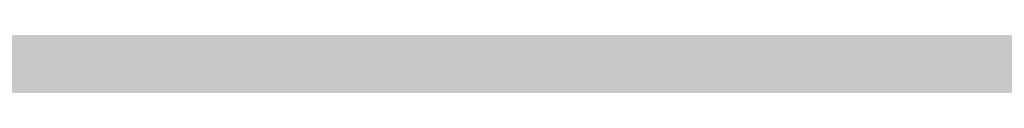
# Model space of a CAD drawing. Units: inches. Extents: x 2091 to 2899, y 967 to 2217.
# Tile 185 of 256: x 2203.16122 to 2203.18039, y 1152.2479 to 1152.24874. Entities that reach past the tile are written whole.
import ezdxf

# ---------------------------------------------------------------- set-up
doc = ezdxf.new("R2010")
doc.units = ezdxf.units.IN
doc.layers.add('A-WALL-PATT', color=141, linetype='Continuous', lineweight=13, true_color=0xadddf7)

msp = doc.modelspace()

# ---------------------------------------------------------------- hatches: boundary and pattern name
at = {"layer": 'A-WALL-PATT'}
h = msp.add_hatch(color=256, dxfattribs=at)
h.dxf.hatch_style = 1
h.paths.add_polyline_path([(2803.143603, 2050.919059), (2203.143603, 2050.919059), (2203.143603, 1090.919059), (2803.143603, 1090.919059)])
h.paths.add_polyline_path([(2635.79885, 1147.540465), (2674.524052, 1147.540465, 0.376086), (2678.529665, 1152.880202), (2678.529665, 1159.556473, 0.333335), (2674.524319, 1163.561846), (2674.524319, 1163.56185), (2674.524319, 1192.93439), (2635.805971, 1192.93439), (2597.087622, 1192.93439), (2597.087622, 1163.561846, 0.333335), (2593.082276, 1159.556473), (2593.082276, 1152.880202, 0.376086), (2597.087889, 1147.540465)], flags=0)
h.paths.add_polyline_path([(2436.010433, 1278.240778, 0.000483), (2435.952643, 1278.215027, -0.001328), (2435.935625, 1278.111693, -0.001711), (2436.11644, 1278.040758, 0.002185)], flags=0)
h.paths.add_polyline_path([(2794.143603, 1143.419059), (2794.143603, 1347.419059), (2543.370171, 1347.419059), (2543.370171, 1351.919059), (2794.143603, 1351.919059), (2794.143603, 1392.713555), (2793.947398, 1392.713555), (2793.947398, 1473.5369), (2794.143603, 1473.5369), (2794.143603, 1531.919059), (2650.143603, 1531.919059), (2650.143603, 1536.419059), (2794.143603, 1536.419059), (2794.143603, 1692.419059), (2609.375609, 1692.419059), (2609.375609, 1644.419059), (2604.875609, 1644.419059), (2604.875609, 1744.919059), (2609.375609, 1744.919059), (2609.375609, 1696.919059), (2794.143603, 1696.919059), (2794.143603, 1780.919059), (2609.643603, 1780.919059), (2493.875609, 1780.919059), (2493.875609, 1785.419059), (2609.643603, 1785.419059), (2794.143603, 1785.419059), (2794.143603, 1847.938821), (2793.951222, 1847.938821), (2793.951222, 1928.762166), (2794.143603, 1928.762166), (2794.143603, 1941.419059), (2614.143603, 1941.419059), (2614.143603, 1821.419059), (2609.643603, 1821.419059), (2609.643603, 1941.419059), (2392.143603, 1941.419059), (2392.143603, 1819.919059), (2387.643603, 1819.919059), (2387.643603, 1941.419059), (2212.143603, 1941.419059), (2212.143603, 1783.919059), (2392.143603, 1783.919059), (2392.143603, 1780.919059), (2212.143603, 1780.919059), (2212.143603, 1629.419059), (2387.643603, 1629.419059), (2387.643603, 1744.919059), (2392.143603, 1744.919059), (2392.143603, 1627.919059), (2317.143603, 1627.919059), (2317.143603, 1551.419059), (2317.143603, 1536.419059), (2459.383591, 1536.419059), (2459.383591, 1602.39648), (2463.883591, 1602.39648), (2463.883591, 1531.919059), (2456.643603, 1531.919059), (2456.643603, 1529.919059), (2452.143603, 1529.919059), (2452.143603, 1531.919059), (2312.643603, 1531.919059), (2312.643603, 1551.419059), (2306.143603, 1551.419059), (2306.143603, 1555.919059), (2308.143603, 1555.919059), (2308.143603, 1551.419059), (2312.643603, 1551.419059), (2312.643603, 1627.919059), (2212.143603, 1627.919059), (2212.143603, 1555.919059), (2270.143603, 1555.919059), (2270.143603, 1551.419059), (2212.143603, 1551.419059), (2212.143603, 1351.919059), (2272.143603, 1351.919059), (2272.143603, 1347.419059), (2212.143603, 1347.419059), (2212.143603, 1275.419059), (2308.143603, 1275.419059), (2308.143603, 1351.919059), (2452.143603, 1351.919059), (2452.143603, 1493.919059), (2456.643603, 1493.919059), (2456.643603, 1347.419059), (2312.643603, 1347.419059), (2312.643603, 1270.919059), (2212.143603, 1270.919059), (2212.143603, 1099.919059), (2281.237523, 1099.919059), (2282.871041, 1110.913803), (2282.008341, 1116.996603), (2278.557741, 1121.420403), (2268.205641, 1128.056203), (2272.087641, 1128.056203), (2273.812941, 1131.927003), (2279.420341, 1134.691903), (2285.027841, 1135.244903), (2287.615841, 1137.456803), (2288.047141, 1138.009803), (2289.341141, 1140.774703), (2291.066541, 1139.668703), (2292.360541, 1135.244903), (2295.379841, 1136.903803), (2296.242541, 1135.797903), (2297.105241, 1133.033003), (2300.124641, 1138.009803), (2303.143941, 1138.009803), (2304.437941, 1135.797903), (2303.143941, 1133.586003), (2306.594641, 1134.691903), (2307.888741, 1133.033003), (2310.908041, 1135.244903), (2313.927441, 1134.138903), (2315.62686, 1132.427102), (2308.320041, 1117.549603), (2290.203841, 1109.807903), (2288.909841, 1103.172103), (2289.272309, 1099.919059), (2434.918227, 1099.919059), (2431.593227, 1124.788059), (2429.930227, 1169.553059), (2430.927185, 1240.519694), (2435.658926, 1238.186126), (2437.135227, 1196.554059), (2438.798227, 1143.973059), (2442.678227, 1111.998059), (2446.558227, 1099.919059), (2794.143603, 1099.919059), (2794.143603, 1138.919059), (2548.032447, 1138.919059), (2548.032447, 1143.419059), (2548.032447, 1148.819059), (2546.668457, 1148.031559), (2528.685692, 1179.178622, 0.256256), (2512.032447, 1148.819059), (2512.032447, 1143.419059), (2512.032447, 1138.919059), (2507.532447, 1138.919059), (2507.532447, 1143.419059), (2507.532447, 1148.819059, 0.256256), (2490.879202, 1179.178622), (2472.896437, 1148.031559), (2471.532447, 1148.819059), (2471.532447, 1143.419059), (2467.032447, 1143.419059), (2467.032447, 1269.945786, 0.039061), (2460.909987, 1273.580059), (2467.032447, 1273.580059), (2467.032447, 1286.325364, 0.014511), (2465.216194, 1286.761905), (2467.032447, 1287.052576), (2467.032447, 1323.419059), (2471.532447, 1323.419059), (2471.532447, 1148.819059), (2489.532447, 1179.995973), (2490.896437, 1179.208473), (2490.879202, 1179.178622, -0.256256), (2507.532447, 1148.819059), (2507.532447, 1143.419059), (2512.032447, 1143.419059), (2512.032447, 1148.819059, -0.256256), (2528.685692, 1179.178622), (2528.668457, 1179.208473), (2530.032447, 1179.995973), (2548.032447, 1148.819059), (2548.032447, 1143.419059)], flags=16)
h.paths.add_polyline_path([(2607.768546, 1200.945083), (2607.768546, 1265.030625), (2597.087622, 1281.052011), (2619.784585, 1281.052011), (2627.795278, 1337.12686), (2635.79885, 1337.12686), (2643.816663, 1337.12686), (2651.827356, 1281.052011), (2674.524319, 1281.052011), (2663.843395, 1265.030625), (2663.843395, 1200.945083), (2635.805971, 1200.945083)], flags=0)
edge = h.paths.add_edge_path(flags=0)
edge.add_ellipse((13303.896215, 1272.998725), major_axis=(-10595.31304, 0.000001), ratio=0.842303870086, start_angle=0.6282372191, end_angle=0.6465540999, ccw=False)
edge.add_ellipse((2711.70045, 1156.852678), major_axis=(2.219769, 0), ratio=0.84230387, start_angle=111.535244, end_angle=180.628237, ccw=False)
edge.add_ellipse((13303.156292, 1272.998725), major_axis=(-10593.026306, 0), ratio=0.842303869544, start_angle=0.5282714718, end_angle=0.6465540971, ccw=False)
edge.add_line((2710.764596, 1175.333295), (2710.129986, 1175.333295))
edge.add_ellipse((2710.129986, 1176.579775), major_axis=(1.479846, 0), ratio=0.84230387, start_angle=180, end_angle=270, ccw=False)
edge.add_line((2708.65014, 1176.579775), (2708.65014, 1200.782914))
edge.add_ellipse((2710.129986, 1200.782914), major_axis=(1.479846, 0), ratio=0.84230387, start_angle=90, end_angle=180, ccw=False)
edge.add_line((2710.129986, 1202.029394), (2710.465075, 1202.029394))
edge.add_ellipse((13303.156292, 1272.998725), major_axis=(-10593.026306, 0), ratio=0.842303869544, start_angle=-0.0902290886, end_angle=0.3838667788, ccw=False)
edge.add_ellipse((2710.129986, 1290.927031), major_axis=(-1.479846, 0), ratio=0.84230387, start_angle=0, end_angle=90, ccw=False)
edge.add_line((2708.65014, 1290.927031), (2708.65014, 1315.13017))
edge.add_ellipse((2710.129986, 1315.13017), major_axis=(-1.479846, 0), ratio=0.84230387, start_angle=-90, end_angle=0, ccw=False)
edge.add_line((2710.129986, 1316.37665), (2710.706314, 1316.37665))
edge.add_ellipse((3238.40172, 1296.289566), major_axis=(528.234, 0), ratio=0.8423038695, start_angle=176.34957241, end_angle=177.82004969, ccw=False)
edge.add_ellipse((2775.063043, 1071.450696), major_axis=(313.307761, 0), ratio=0.8423038695, start_angle=102.12596555, end_angle=103.78052899, ccw=False)
edge.add_ellipse((2775.063043, 1078.305698), major_axis=(-305.302891, 0), ratio=0.8423038695, start_angle=-79.790461, end_angle=-77.55537271, ccw=False)
edge.add_ellipse((2695.141767, 1541.975383), major_axis=(-250.960216, 0), ratio=0.8423038695, start_angle=99.25656601, end_angle=102.55493264)
edge.add_line((2741.410326, 1334.214255), (2747.132545, 1337.378477))
edge.add_ellipse((2747.538616, 1336.857478), major_axis=(-0.739923, 0), ratio=0.8423039, start_angle=270, end_angle=307.93313, ccw=False)
edge.add_ellipse((2747.538616, 1336.857478), major_axis=(-0.739923, 0), ratio=0.8423039, start_angle=232.06687, end_angle=270, ccw=False)
edge.add_line((2747.944687, 1337.378477), (2753.666906, 1334.214255))
edge.add_ellipse((2799.935466, 1541.975383), major_axis=(250.960216, 0), ratio=0.8423038695, start_angle=257.44506736, end_angle=260.74343399)
edge.add_ellipse((2720.014189, 1078.305698), major_axis=(305.302891, 0), ratio=0.8423038695, start_angle=77.55537271, end_angle=79.790461, ccw=False)
edge.add_ellipse((2720.014189, 1071.450696), major_axis=(-313.307761, 0), ratio=0.8423038695, start_angle=256.21947101, end_angle=257.87403445, ccw=False)
edge.add_ellipse((2256.675512, 1296.289566), major_axis=(-528.234, 0), ratio=0.8423038695, start_angle=182.17995031, end_angle=183.65042759, ccw=False)
edge.add_line((2784.370918, 1316.37665), (2784.947247, 1316.37665))
edge.add_ellipse((2784.947247, 1315.13017), major_axis=(1.479846, 0), ratio=0.84230387, start_angle=0, end_angle=90, ccw=False)
edge.add_line((2786.427093, 1315.13017), (2786.427093, 1290.927031))
edge.add_ellipse((2784.947247, 1290.927031), major_axis=(1.479846, 0), ratio=0.84230387, start_angle=270, end_angle=360, ccw=False)
edge.add_ellipse((-7808.07906, 1272.998725), major_axis=(10593.026306, 0), ratio=0.842303869544, start_angle=-0.3838667788, end_angle=0.0902290886, ccw=False)
edge.add_line((2784.612157, 1202.029394), (2784.947247, 1202.029394))
edge.add_ellipse((2784.947247, 1200.782914), major_axis=(1.479846, 0), ratio=0.84230387, start_angle=0, end_angle=90, ccw=False)
edge.add_line((2786.427093, 1200.782914), (2786.427093, 1176.579775))
edge.add_ellipse((2784.947247, 1176.579775), major_axis=(-1.479846, 0), ratio=0.84230387, start_angle=90, end_angle=180, ccw=False)
edge.add_line((2784.947247, 1175.333295), (2784.312636, 1175.333295))
edge.add_ellipse((-7808.07906, 1272.998725), major_axis=(10593.026306, 0), ratio=0.842303869544, start_angle=-0.6186431963, end_angle=-0.5282714718, ccw=False)
edge.add_ellipse((2783.376783, 1156.852678), major_axis=(-2.219769, 0), ratio=0.84230387, start_angle=179.371763, end_angle=248.464757, ccw=False)
edge.add_ellipse((-7808.818983, 1272.998725), major_axis=(-10595.31304, 0.000004), ratio=0.842303865762, start_angle=179.3534459226, end_angle=179.3717628034, ccw=False)
edge.add_ellipse((2780.297303, 1153.500793), major_axis=(-5.246426, 0), ratio=0.84230387, start_angle=90, end_angle=179.353446, ccw=False)
edge.add_line((2780.297303, 1149.081708), (2714.77993, 1149.081708))
edge.add_ellipse((2714.77993, 1153.500793), major_axis=(5.246426, 0), ratio=0.84230387, start_angle=180.646554, end_angle=270, ccw=False)
edge = h.paths.add_edge_path(flags=0)
edge.add_line((2718.187367, 1151.007833), (2718.187367, 1170.472364))
edge.add_ellipse((2721.14706, 1170.472364), major_axis=(-2.959692, 0), ratio=0.84230387, start_angle=-90, end_angle=0, ccw=False)
edge.add_line((2721.14706, 1172.965324), (2773.930173, 1172.965324))
edge.add_ellipse((2773.930173, 1170.472364), major_axis=(-2.959692, 0), ratio=0.84230387, start_angle=180, end_angle=270, ccw=False)
edge.add_line((2776.889865, 1170.472364), (2776.889865, 1151.007833))
edge.add_line((2776.889865, 1151.007833), (2718.187367, 1151.007833))
edge = h.paths.add_edge_path(flags=0)
edge.add_line((2718.187367, 1180.23415), (2718.187367, 1199.057834))
edge.add_ellipse((2747.538616, 1320.39864), major_axis=(147.017924, 0), ratio=0.8423038695, start_angle=256.40186531, end_angle=283.59813469)
edge.add_line((2776.889865, 1199.057834), (2776.889865, 1180.23415))
edge.add_ellipse((2747.538616, 1301.574956), major_axis=(147.017924, 0), ratio=0.8423038695, start_angle=256.40186531, end_angle=283.59813469, ccw=False)
edge = h.paths.add_edge_path(flags=0)
edge.add_ellipse((13303.156292, 1272.998725), major_axis=(-10591.54646, 0), ratio=0.842303869555, start_angle=0.0555943135, end_angle=0.3777641939, ccw=False)
edge.add_line((2711.616859, 1262.72171), (2715.667408, 1249.495396))
edge.add_ellipse((6413.891963, 1241.691919), major_axis=(-3698.236159, 0), ratio=0.84230386955, start_angle=-0.120897369, end_angle=0.364076349)
edge.add_line((2715.761038, 1218.192455), (2711.934307, 1203.167361))
edge = h.paths.add_edge_path(flags=0)
edge.add_line((2718.187367, 1251.074566), (2716.002485, 1267.450435))
edge.add_ellipse((2742.151175, 1202.18954), major_axis=(81.772585, 0), ratio=0.84230387, start_angle=94.27742096, end_angle=111.8349538, ccw=False)
edge.add_line((2737.009748, 1270.930626), (2758.067484, 1270.930626))
edge.add_ellipse((2752.926058, 1202.18954), major_axis=(81.772585, 0), ratio=0.84230387, start_angle=68.1650462, end_angle=85.72257904, ccw=False)
edge.add_line((2779.074747, 1267.450435), (2776.889865, 1251.074566))
edge.add_ellipse((2750.338059, 1187.885356), major_axis=(79.579664, 0), ratio=0.84230387, start_angle=67.20808512, end_angle=85.1299304)
edge.add_line((2756.034656, 1254.743656), (2739.042576, 1254.743656))
edge.add_ellipse((2744.739174, 1187.885356), major_axis=(79.579664, 0), ratio=0.84230387, start_angle=94.8700696, end_angle=112.79191488)
edge = h.paths.add_edge_path(flags=0)
edge.add_line((2783.142926, 1203.167361), (2779.316194, 1218.192455))
edge.add_ellipse((-918.81473, 1241.691919), major_axis=(3698.236159, 0), ratio=0.84230386955, start_angle=-0.364076349, end_angle=0.120897369)
edge.add_line((2779.409825, 1249.495396), (2783.460373, 1262.72171))
edge.add_ellipse((-7808.07906, 1272.998725), major_axis=(-10591.54646, 0), ratio=0.84230386954, start_angle=179.6222358061, end_angle=179.9444056865, ccw=False)
edge = h.paths.add_edge_path(flags=0)
edge.add_ellipse((2734.200892, 1286.69044), major_axis=(-0.356609, 6.340078), ratio=0.60383358, start_angle=89.0020143, end_angle=253.657408, ccw=False)
edge.add_line((2730.369001, 1286.541806), (2730.369001, 1301.35198))
edge.add_line((2730.369001, 1301.35198), (2735.913311, 1305.214803))
edge.add_ellipse((2736.384917, 1304.734561), major_axis=(0.739923, 0), ratio=0.8423039, start_angle=90, end_angle=134.480211, ccw=False)
edge.add_line((2736.384917, 1305.357801), (2738.032783, 1305.357801))
edge.add_line((2738.032783, 1305.357801), (2738.032783, 1307.707927))
edge.add_ellipse((2794.201642, 1307.707927), major_axis=(56.168859, 0), ratio=0.84230387, start_angle=150.5614304, end_angle=180, ccw=False)
edge.add_ellipse((2700.875591, 1307.707927), major_axis=(-56.168859, 0), ratio=0.84230387, start_angle=180, end_angle=209.4385696, ccw=False)
edge.add_line((2757.04445, 1307.707927), (2757.04445, 1305.357801))
edge.add_line((2757.04445, 1305.357801), (2758.692316, 1305.357801))
edge.add_ellipse((2758.692316, 1304.734561), major_axis=(-0.739923, 0), ratio=0.8423039, start_angle=225.519789, end_angle=270, ccw=False)
edge.add_line((2759.163922, 1305.214803), (2764.708231, 1301.35198))
edge.add_line((2764.708231, 1301.35198), (2764.708231, 1286.541806))
edge.add_ellipse((2760.87634, 1286.69044), major_axis=(0.356609, 6.340078), ratio=0.60383358, start_angle=106.342592, end_angle=270.9979857, ccw=False)
edge.add_line((2757.04445, 1285.79709), (2757.04445, 1307.707927))
edge.add_ellipse((2700.875591, 1307.707927), major_axis=(-56.168859, 0), ratio=0.84230387, start_angle=180, end_angle=209.4385696)
edge.add_ellipse((2794.201642, 1307.707927), major_axis=(56.168859, 0), ratio=0.84230387, start_angle=150.5614304, end_angle=180)
edge.add_line((2738.032783, 1307.707927), (2738.032783, 1285.79709))
h.paths.add_polyline_path([(2417.812273, 1104.449704), (2413.492273, 1102.529704), (2410.612273, 1103.969704), (2409.172273, 1106.369704), (2407.252273, 1107.329704), (2406.292273, 1109.729704), (2405.332273, 1114.049704), (2405.332273, 1117.889704), (2406.292273, 1120.129704), (2407.252273, 1119.809704), (2408.848322, 1118.327658), (2410.173945, 1119.42417), (2410.211273, 1120.405704), (2411.040731, 1121.419054), (2410.699273, 1119.858704), (2410.173945, 1119.42417), (2410.088452, 1117.176109), (2411.132836, 1116.206324), (2413.972273, 1119.329704), (2416.852273, 1120.769704), (2416.869721, 1120.798784), (2417.035071, 1119.405116), (2417.896213, 1118.143384), (2418.292273, 1118.369704), (2419.544447, 1120.039269), (2419.360915, 1118.387487), (2419.032108, 1119.356151), (2418.398939, 1118.511926), (2419.252273, 1114.529704), (2418.794091, 1107.198795)], flags=0)
h.paths.add_polyline_path([(2508.870171, 1347.419059), (2508.370171, 1347.419059), (2508.370171, 1351.919059), (2508.870171, 1351.919059)], flags=0)
h.paths.add_polyline_path([(2473.370171, 1347.419059), (2472.370171, 1347.419059), (2467.870171, 1347.419059), (2467.870171, 1455.419059), (2472.370171, 1455.419059), (2472.370171, 1352.419059), (2473.370171, 1352.419059)], flags=0)
h.paths.add_polyline_path([(2352.106244, 1217.446197), (2349.226244, 1218.886197), (2347.786244, 1221.286197), (2345.866244, 1222.246197), (2344.906244, 1224.646197), (2343.946244, 1228.966197), (2343.946244, 1232.806197), (2344.906244, 1235.046197), (2345.866244, 1234.726197), (2347.462293, 1233.244152), (2348.787916, 1234.340663), (2348.825244, 1235.322197), (2349.654702, 1236.335547), (2349.313244, 1234.775197), (2348.787916, 1234.340663), (2348.702423, 1232.092603), (2349.746807, 1231.122817), (2352.586244, 1234.246197), (2355.466244, 1235.686197), (2355.483692, 1235.715277), (2355.649043, 1234.321609), (2356.510185, 1233.059877), (2356.906244, 1233.286197), (2358.158418, 1234.955762), (2357.974887, 1233.30398), (2357.646079, 1234.272644), (2357.012911, 1233.428419), (2357.866244, 1229.446197), (2357.408062, 1222.115288), (2356.426244, 1219.366197)], flags=0)
h.paths.add_polyline_path([(2348.2968, 1112.22442), (2347.0138, 1112.31042), (2345.5298, 1114.12742), (2345.7318, 1115.85842), (2346.8118, 1116.98242), (2346.8118, 1114.64642), (2345.8668, 1114.21442), (2346.8798, 1114.30042)], flags=0)
h.paths.add_polyline_path([(2347.0138, 1110.92642), (2346.2718, 1110.49342), (2346.6098, 1111.18642)], flags=0)
h.paths.add_polyline_path([(2345.8668, 1118.19442), (2345.5298, 1117.32942), (2343.7078, 1118.02142), (2344.3828, 1118.62642)], flags=0)
h.paths.add_polyline_path([(2346.6768, 1109.28242), (2346.0698, 1108.07142), (2345.8668, 1110.06142)], flags=0)
h.paths.add_polyline_path([(2345.0568, 1119.75142), (2343.6398, 1119.75142), (2343.9778, 1121.13542)], flags=0)
h.paths.add_polyline_path([(2345.2598, 1116.55042), (2345.1248, 1115.85842), (2344.9218, 1115.68542), (2344.7198, 1116.37742)], flags=0)
h.paths.add_polyline_path([(2345.6648, 1112.31042), (2345.4618, 1111.53242), (2344.0448, 1111.96442), (2344.6518, 1112.57042)], flags=0)
h.paths.add_polyline_path([(2345.1918, 1113.34942), (2344.4498, 1113.86842), (2344.7198, 1114.38742)], flags=0)
h.paths.add_polyline_path([(2344.6518, 1116.80942), (2344.1798, 1115.68542), (2344.6518, 1115.33942), (2343.9098, 1114.90642), (2343.0328, 1115.94442), (2343.6398, 1116.46342)], flags=0)
h.paths.add_polyline_path([(2345.8668, 1106.68642), (2344.9898, 1105.56242), (2344.5168, 1106.60042)], flags=0)
h.paths.add_polyline_path([(2344.8548, 1110.06142), (2344.5168, 1109.28242), (2344.1128, 1109.71542)], flags=0)
h.paths.add_polyline_path([(2344.0448, 1113.52242), (2343.4378, 1113.08942), (2342.7628, 1113.95442)], flags=0)
h.paths.add_polyline_path([(2344.3148, 1111.01242), (2342.9648, 1110.32042), (2342.9648, 1111.09942)], flags=0)
h.paths.add_polyline_path([(2345.1248, 1104.69742), (2344.5848, 1103.74542), (2344.4498, 1104.26442)], flags=0)
h.paths.add_polyline_path([(2342.8298, 1121.22242), (2341.7498, 1120.53042), (2340.5358, 1121.04942), (2340.1308, 1121.82842), (2340.6708, 1122.95242), (2341.1428, 1121.82842), (2341.6148, 1122.00142)], flags=0)
h.paths.add_polyline_path([(2342.9648, 1119.75142), (2343.0328, 1118.45342), (2342.0878, 1118.02142), (2342.0198, 1119.49142)], flags=0)
h.paths.add_polyline_path([(2342.6948, 1116.89642), (2341.9528, 1116.63642), (2342.0198, 1117.32942)], flags=0)
h.paths.add_polyline_path([(2343.0328, 1112.22442), (2342.0198, 1111.79142), (2341.5478, 1112.22442), (2342.3578, 1113.34942)], flags=0)
h.paths.add_polyline_path([(2343.7748, 1104.43742), (2342.6278, 1102.88042), (2342.6948, 1104.61042), (2343.4378, 1105.12942)], flags=0)
h.paths.add_polyline_path([(2342.0198, 1115.07942), (2340.8058, 1115.51242), (2340.9408, 1116.37742)], flags=0)
h.paths.add_polyline_path([(2341.4808, 1120.09742), (2341.4808, 1119.40542), (2341.0758, 1119.57842), (2341.1428, 1120.09742)], flags=0)
h.paths.add_polyline_path([(2341.8178, 1114.47342), (2340.9408, 1113.08942), (2340.8058, 1114.56042)], flags=0)
h.paths.add_polyline_path([(2341.1428, 1118.54042), (2340.9408, 1116.98242), (2339.0508, 1117.67542), (2339.0508, 1118.62642)], flags=0)
h.paths.add_polyline_path([(2342.6948, 1101.66842), (2341.9528, 1101.84142), (2342.5598, 1102.36142)], flags=0)
h.paths.add_polyline_path([(2340.3328, 1119.66542), (2338.4438, 1119.57842), (2337.9038, 1120.35742), (2339.6578, 1120.61642)], flags=0)
h.paths.add_polyline_path([(2340.3328, 1115.33942), (2340.0628, 1113.69542), (2339.3878, 1115.33942)], flags=0)
h.paths.add_polyline_path([(2341.8178, 1103.83142), (2341.5478, 1102.88042), (2341.1428, 1103.65842)], flags=0)
h.paths.add_polyline_path([(2339.0508, 1122.86642), (2337.2958, 1121.82842), (2337.0938, 1123.12542), (2337.7688, 1123.81842)], flags=0)
h.paths.add_polyline_path([(2339.1178, 1121.74142), (2338.8478, 1121.22242), (2338.1738, 1121.04942), (2338.3758, 1121.56842)], flags=0)
h.paths.add_polyline_path([(2339.1858, 1119.31942), (2338.6458, 1118.71342), (2338.2408, 1118.10742), (2338.2408, 1118.88642)], flags=0)
h.paths.add_polyline_path([(2341.1428, 1101.92842), (2340.6028, 1101.23642), (2340.0628, 1101.84142), (2340.6028, 1102.36142)], flags=0)
h.paths.add_polyline_path([(2337.6338, 1117.76142), (2336.6208, 1118.28042), (2337.2958, 1118.97242)], flags=0)
h.paths.add_polyline_path([(2336.8238, 1119.57842), (2334.7988, 1118.97242), (2335.2038, 1120.35742), (2336.5538, 1120.87642)], flags=0)
h.paths.add_polyline_path([(2339.1178, 1100.45742), (2337.3638, 1100.54342), (2336.7558, 1101.23642)], flags=0)
h.paths.add_polyline_path([(2336.3508, 1122.43342), (2336.0138, 1121.91442), (2334.9338, 1122.43342), (2334.5288, 1123.47142), (2335.7438, 1122.77942)], flags=0)
h.paths.add_polyline_path([(2334.7318, 1120.87642), (2334.2588, 1120.35742), (2334.0568, 1120.78942), (2334.5968, 1121.30842)], flags=0)
h.paths.add_polyline_path([(2334.4618, 1122.17442), (2332.5718, 1121.30842), (2331.3568, 1122.17442), (2332.0998, 1122.86642)], flags=0)
h.paths.add_polyline_path([(2334.2588, 1118.54042), (2333.3818, 1118.45342), (2333.6518, 1119.31942)], flags=0)
h.paths.add_polyline_path([(2335.5418, 1102.27442), (2334.1918, 1102.62042), (2335.2718, 1103.31242)], flags=0)
h.paths.add_polyline_path([(2332.7068, 1119.66542), (2331.6948, 1120.44342), (2332.5048, 1120.78942)], flags=0)
h.paths.add_polyline_path([(2334.7318, 1101.14942), (2333.5168, 1101.58242), (2333.9888, 1101.75542)], flags=0)
h.paths.add_polyline_path([(2332.6398, 1116.63642), (2331.0868, 1116.29042), (2331.9648, 1118.19442)], flags=0)
h.paths.add_polyline_path([(2330.7498, 1121.56842), (2330.2768, 1120.27042), (2328.5228, 1119.31942), (2328.9948, 1121.04942)], flags=0)
h.paths.add_polyline_path([(2330.7498, 1118.62642), (2330.0078, 1117.50242), (2329.8728, 1118.02142)], flags=0)
h.paths.add_polyline_path([(2332.0998, 1102.36142), (2330.5468, 1102.01442), (2331.6948, 1102.96642)], flags=0)
h.paths.add_polyline_path([(2329.5348, 1113.60842), (2329.0628, 1112.31042), (2328.5898, 1113.34942)], flags=0)
h.paths.add_polyline_path([(2328.3878, 1117.84842), (2327.5098, 1116.55042), (2327.1728, 1117.76142)], flags=0)
h.paths.add_polyline_path([(2329.7378, 1106.51342), (2329.5348, 1105.30242), (2328.2528, 1106.08142)], flags=0)
h.paths.add_polyline_path([(2328.6578, 1114.38742), (2328.0498, 1114.12742), (2328.3198, 1114.90642)], flags=0)
h.paths.add_polyline_path([(2328.3198, 1112.22442), (2327.1058, 1112.13742), (2326.7008, 1112.65642)], flags=0)
h.paths.add_polyline_path([(2326.9028, 1115.25242), (2326.7008, 1114.12742), (2325.2158, 1113.60842), (2326.0928, 1115.33942)], flags=0)
h.paths.add_polyline_path([(2326.6328, 1108.33042), (2326.0928, 1107.37942), (2325.8908, 1108.50342), (2326.4978, 1109.10942)], flags=0)
h.paths.add_polyline_path([(2615.143603, 1531.919059), (2609.643603, 1531.919059), (2609.643603, 1620.419059), (2614.143603, 1620.419059), (2614.143603, 1536.419059), (2615.143603, 1536.419059)], flags=0)
h.paths.add_polyline_path([(2545.143603, 1563.419059), (2464.143603, 1563.419059), (2464.143603, 1632.419059), (2509.143603, 1632.419059), (2509.143603, 1627.919059), (2509.143603, 1603.919059), (2468.643603, 1603.919059), (2468.643603, 1567.919059), (2540.643603, 1567.919059), (2540.643603, 1591.919059), (2545.143603, 1591.919059)], flags=0)
h.paths.add_polyline_path([(2388.969048, 1549.985735), (2357.434181, 1549.985735), (2357.434181, 1623.360778), (2399.362777, 1623.360778), (2435.689465, 1623.360778), (2435.592547, 1602.559273), (2435.592547, 1602.39648), (2388.969048, 1602.39648)], flags=0)
h.paths.add_polyline_path([(2388.880628, 1555.809151), (2374.904429, 1555.809151), (2374.904429, 1600.571564), (2374.904429, 1615.457645), (2406.350877, 1615.457645), (2406.350877, 1618.939431), (2412.174293, 1615.457645), (2406.350877, 1611.97586), (2406.350877, 1615.457645), (2388.880628, 1615.457645)], flags=0)
h.paths.add_polyline_path([(2568.875609, 1644.419059), (2453.375609, 1644.419059), (2453.375609, 1785.419059), (2457.875609, 1785.419059), (2457.875609, 1648.919059), (2568.875609, 1648.919059)], flags=0)
h.paths.add_polyline_path([(2212.143603, 1945.919059), (2212.143603, 2041.919059), (2794.143603, 2041.919059), (2794.143603, 1945.919059)], flags=16)
h.paths.add_polyline_path([(2271.082728, 1964.317238), (2776.852968, 1964.317238), (2776.852968, 2037.169623), (2271.082728, 2037.169623)], flags=8)
h.paths.add_polyline_path([(2380.649285, 1536.824144), (2461.040809, 1536.824144), (2461.040809, 1554.652587), (2380.649285, 1554.652587)], flags=8)
h.paths.add_polyline_path([(2240.755709, 1609.725451), (2309.185829, 1609.725451), (2309.185829, 1617.698204), (2240.755709, 1617.698204)], flags=8)
h.paths.add_polyline_path([(2212.677255, 1313.504102), (2282.59152, 1313.504102), (2282.59152, 1322.745239), (2212.677255, 1322.745239)], flags=8)
h.paths.add_polyline_path([(2457.111976, 1114.778574), (2558.481581, 1114.778574), (2558.481581, 1142.219682), (2457.111976, 1142.219682)], flags=8)
h.paths.add_polyline_path([(2473.442337, 1273.010067), (2604.641226, 1273.010067), (2604.641226, 1318.346935), (2473.442337, 1318.346935)], flags=8)
h.paths.add_polyline_path([(2638.876302, 1626.977432), (2684.250367, 1627.976738), (2684.038483, 1637.597494), (2638.664417, 1636.598188)], flags=8)
h.paths.add_polyline_path([(2537.590554, 1453.793447), (2628.389547, 1453.793447), (2628.389547, 1475.344811), (2537.590554, 1475.344811)], flags=8)
h.paths.add_polyline_path([(2504.137638, 1714.632397), (2554.647187, 1714.632397), (2554.647187, 1730.237712), (2504.137638, 1730.237712)], flags=8)
h.paths.add_polyline_path([(2487.501181, 1575.651872), (2535.097121, 1575.651872), (2535.097121, 1598.377646), (2487.501181, 1598.377646)], flags=8)
h.paths.add_polyline_path([(2709.0994, 1735.710278), (2740.016601, 1735.710278), (2740.016601, 1749.937641), (2709.0994, 1749.937641)], flags=8)
h.paths.add_polyline_path([(2442.438424, 1792.171657), (2564.728835, 1792.171657), (2564.728835, 1842.000163), (2442.438424, 1842.000163)], flags=8)
h.paths.add_polyline_path([(2655.815801, 1809.644076), (2789.520142, 1806.693796), (2790.084977, 1832.291638), (2656.380635, 1835.241918)], flags=8)
h.paths.add_polyline_path([(2234.842697, 1797.720143), (2368.592851, 1794.768852), (2369.160718, 1820.504132), (2235.410564, 1823.455423)], flags=8)
h.paths.add_polyline_path([(2245.138466, 1644.006335), (2398.427733, 1640.6239), (2398.994842, 1666.32482), (2245.705575, 1669.707255)], flags=8)
h.paths.add_polyline_path([(2306.142847, 1431.168519), (2413.768314, 1428.793687), (2414.333148, 1454.391529), (2306.707682, 1456.76636)], flags=8)
h.paths.add_polyline_path([(2306.834582, 1458.233145), (2393.380484, 1456.323449), (2393.932808, 1481.354358), (2307.386907, 1483.264054)], flags=8)

doc.saveas('drawing.dxf')
